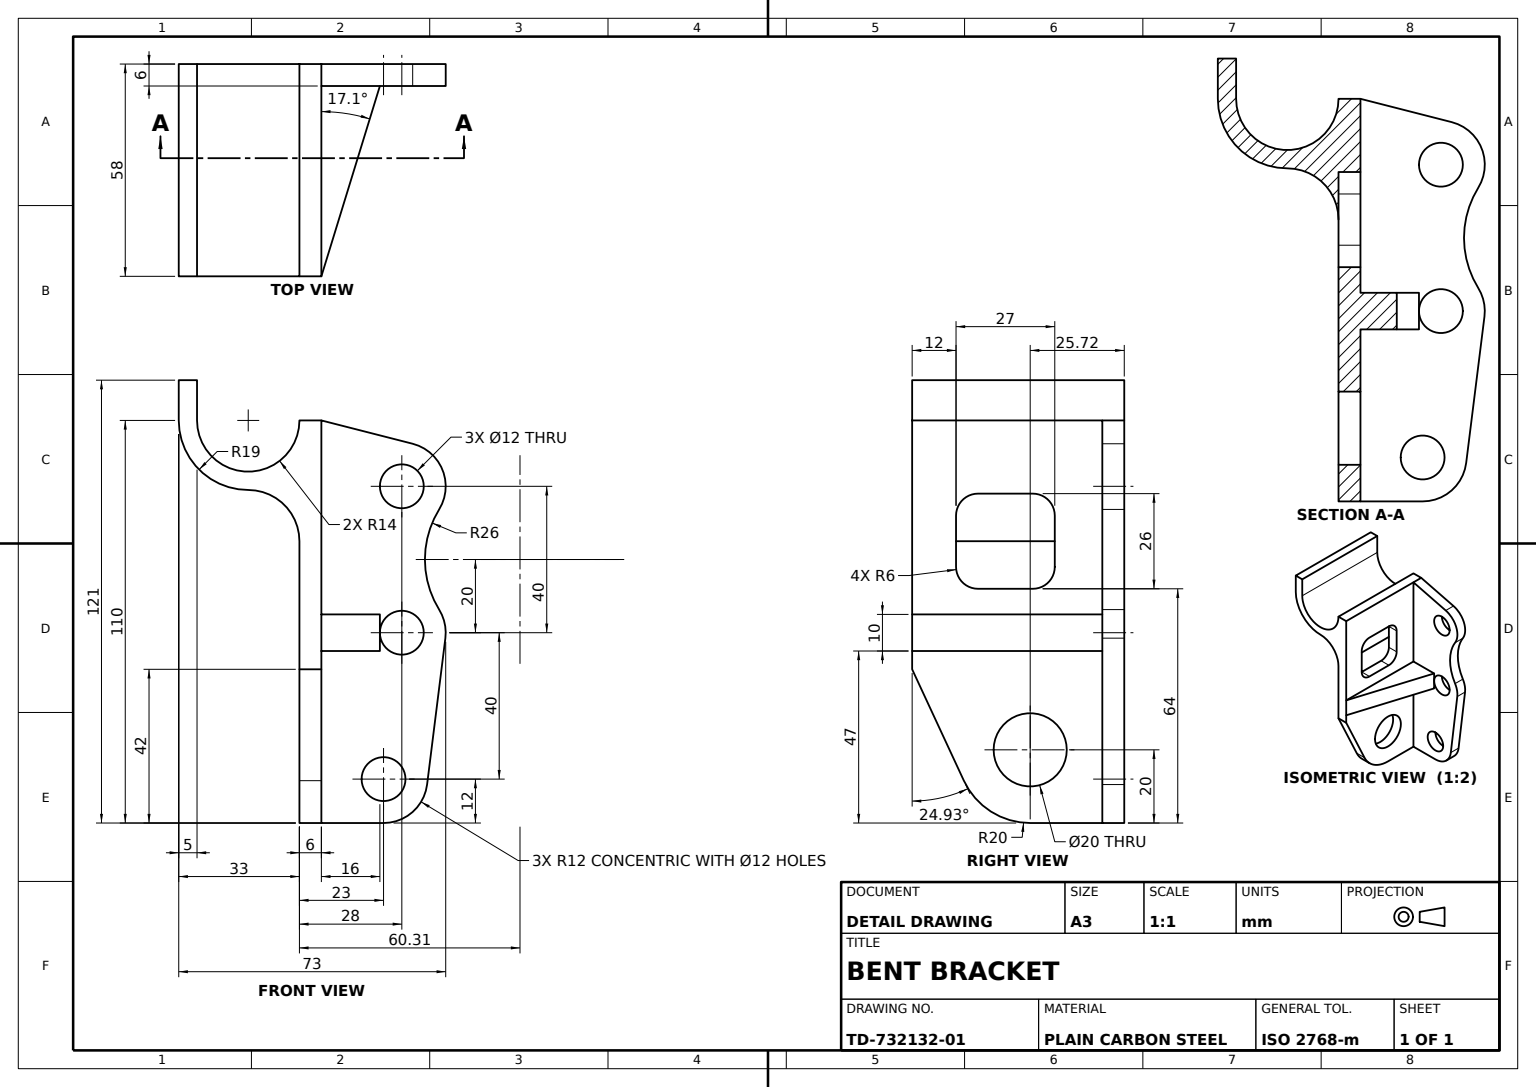
from build123d import *

# Parameters (mm, degrees)
BACK_PLATE_PROFILE_R   = 6
BACK_PLATE_6MM_DEPTH   = 6
SIDE_FLANGE_PROFILE_R  = 10
SIDE_FLANGE_6MM_DEPTH  = 6
GUSSET_RIB_10MM_REACH  = 93.258
GUSSET_RIB_PATH_WALL_W = 238.92163478
GUSSET_RIB_PATH_WALL_H = 10
CRADLE_SADDLE_REACH    = 132.629


with BuildPart() as part:
    # Back Plate Profile → Back Plate 6mm (new body)
    with BuildSketch(Plane.XY):
        with BuildLine():
            Line((0, 0), (6, 0))
            Line((6, 0), (30.967735953, -6.372767169))
            ThreePointArc((30.967735953, -6.372767169), (39.129158997, -13.512036094), (38.203470161, -24.315789474))
            ThreePointArc((38.203470161, -24.315789474), (34.310988843, -38), (38.203470161, -51.684210526))
            ThreePointArc((38.203470161, -51.684210526), (39.723835971, -55.440376954), (39.907334521, -59.488416815))
            Line((39.907334521, -59.488416815), (34.907334521, -99.488416815))
            ThreePointArc((34.907334521, -99.488416815), (30.941630759, -106.99613811), (23, -110))
            Line((23, -110), (0, -110))
            Line((0, -110), (0, 0))
        make_face()
        with Locations((23, -98)):
            Circle(BACK_PLATE_PROFILE_R, mode=Mode.SUBTRACT)
        with Locations((28, -58)):
            Circle(BACK_PLATE_PROFILE_R, mode=Mode.SUBTRACT)
        with Locations((28, -18)):
            Circle(BACK_PLATE_PROFILE_R, mode=Mode.SUBTRACT)
    extrude(amount=BACK_PLATE_6MM_DEPTH)

    # Side Flange Profile → Side Flange 6mm (add)
    with BuildSketch(Plane(origin=(0, 0, 0), x_dir=(0, 0, -1), z_dir=(1, 0, 0))):
        with BuildLine():
            Line((0, 0), (-58, 0))
            Line((-58, 0), (-58, -68))
            Line((-58, -68), (-43.858565284, -98.428947708))
            ThreePointArc((-43.858565284, -98.428947708), (-36.478390759, -106.860886011), (-25.721508176, -110))
            Line((-25.721508176, -110), (-5.721508176, -110))
            Line((-5.721508176, -110), (0, -110))
            Line((0, -110), (0, 0))
        make_face()
        with Locations((-25.721508176, -90)):
            Circle(SIDE_FLANGE_PROFILE_R, mode=Mode.SUBTRACT)
        with BuildLine():
            Line((-40, -46), (-25, -46))
            ThreePointArc((-25, -46), (-20.757359313, -44.242640687), (-19, -40))
            Line((-19, -40), (-19, -26))
            ThreePointArc((-19, -26), (-20.757359313, -21.757359313), (-25, -20))
            Line((-25, -20), (-40, -20))
            ThreePointArc((-40, -20), (-44.242640687, -21.757359313), (-46, -26))
            Line((-46, -26), (-46, -40))
            ThreePointArc((-46, -40), (-44.242640687, -44.242640687), (-40, -46))
        make_face(mode=Mode.SUBTRACT)
    extrude(amount=SIDE_FLANGE_6MM_DEPTH)

    # Gusset Rib Path wall → Gusset Rib 10mm (add, up to next)
    with BuildSketch(Plane(origin=(14, -58, 32), x_dir=(0.294085848838, 0, -0.955779008722), z_dir=(-0.955779008722, 0, -0.294085848838)), mode=Mode.PRIVATE) as gusset_rib_10mm_sk1:
        Rectangle(GUSSET_RIB_PATH_WALL_W, GUSSET_RIB_PATH_WALL_H)
    gusset_rib_10mm_tool1 = extrude(gusset_rib_10mm_sk1.sketch, amount=GUSSET_RIB_10MM_REACH, mode=Mode.PRIVATE) - part.part
    add(gusset_rib_10mm_tool1.solids().sort_by_distance((14, -58, 32))[0])

    # Cradle Saddle: up to this face of the body (flat: up to its plane)
    cradle_saddle_end = Plane(part.part.faces().sort_by_distance((17.427592869, -55.606488982, 0))[0])
    # Cradle Saddle Profile → Cradle Saddle (add, up to the picked face)
    with BuildSketch(Plane.XY.offset(58), mode=Mode.PRIVATE) as cradle_saddle_sk1:
        with BuildLine():
            Line((-33, 0), (-33, 11))
            Line((-33, 11), (-28, 11))
            Line((-28, 11), (-28, 0))
            ThreePointArc((-28, 0), (-14, -14), (0, 0))
            Line((0, 0), (0, -33))
            ThreePointArc((0, -33), (-4.100505063, -23.100505063), (-14, -19))
            ThreePointArc((-14, -19), (-27.435028843, -13.435028843), (-33, 0))
        make_face()
    cradle_saddle_tool1 = split(extrude(cradle_saddle_sk1.sketch, amount=-CRADLE_SADDLE_REACH, mode=Mode.PRIVATE), bisect_by=cradle_saddle_end, keep=Keep.BOTH, mode=Mode.PRIVATE)
    add(cradle_saddle_tool1.solids().sort_by(Axis((-27.04612, -13.04612, 58), (0, 0, -1)))[0])


solid = part.part
